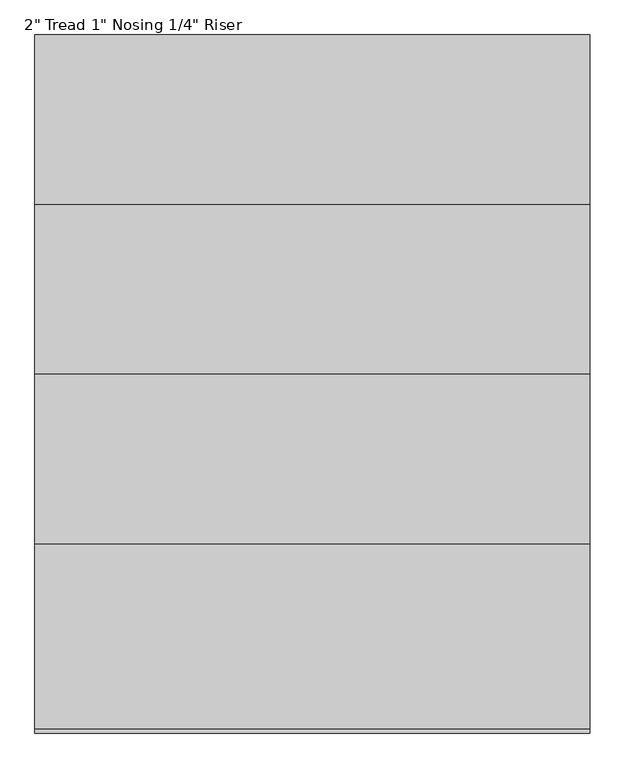
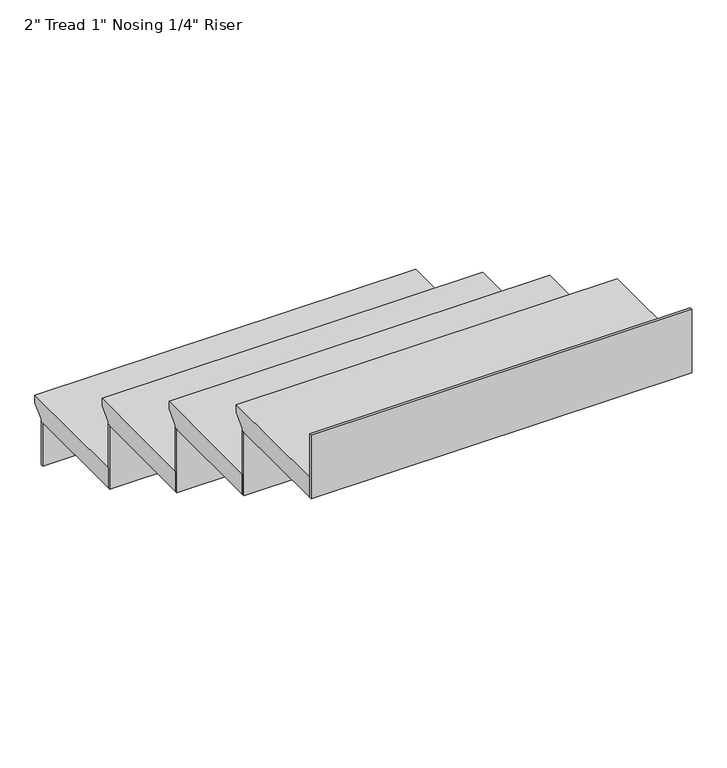
"""IFC4 building model written with IfcOpenShell, lengths in millimetres: stair flight geometry."""

from ifc_helpers import new_model, si_unit, origin, place, context, project, spatial, faceted_brep, source, transform, mapped, element, save


def stair_flight_6dcdbca7(model_context):
    return source(origin(), model_context, "Body", "Brep", [
        faceted_brep([(2695.3430349, 4115.4555142, 1415.3029412), (2695.3430349, 4115.4555142, 1434.3529412), (3609.7430349, 4115.4555142, 1434.3529412), (3609.7430349, 4115.4555142, 1415.3029412), (2695.3430349, 4090.0555142, 1389.9029412), (3609.7430349, 4090.0555142, 1389.9029412), (2695.3430349, 3810.6555142, 1434.3529412), (3609.7430349, 3810.6555142, 1434.3529412), (3609.7430349, 4090.0555142, 1383.5529412), (3609.7430349, 3810.6555142, 1383.5529412), (2695.3430349, 3810.6555142, 1383.5529412), (2695.3430349, 4090.0555142, 1383.5529412)], [[[0, 1, 2, 3]], [[4, 0, 3, 5]], [[2, 1, 6, 7]], [[8, 9, 10, 11]], [[2, 7, 9, 8, 5, 3]], [[8, 11, 4, 5]], [[6, 1, 0, 4, 11, 10]], [[7, 6, 10, 9]]]),
        faceted_brep([(2695.3430349, 4090.0555142, 1383.5529412), (2695.3430349, 4090.0555142, 1272.9882353), (2695.3430349, 4083.7055142, 1272.9882353), (2695.3430349, 4083.7055142, 1383.5529412), (3609.7430349, 4090.0555142, 1383.5529412), (3609.7430349, 4083.7055142, 1383.5529412), (3609.7430349, 4083.7055142, 1272.9882353), (3609.7430349, 4090.0555142, 1272.9882353)], [[[0, 1, 2, 3]], [[4, 5, 6, 7]], [[1, 0, 4, 7]], [[2, 1, 7, 6]], [[3, 2, 6, 5]], [[0, 3, 5, 4]]]),
        faceted_brep([(2695.3430349, 3810.6555142, 1544.9176471), (2695.3430349, 3810.6555142, 1383.5529412), (2695.3430349, 3804.3055142, 1383.5529412), (2695.3430349, 3804.3055142, 1544.9176471), (3609.7430349, 3810.6555142, 1544.9176471), (3609.7430349, 3804.3055142, 1544.9176471), (3609.7430349, 3804.3055142, 1383.5529412), (3609.7430349, 3810.6555142, 1383.5529412)], [[[0, 1, 2, 3]], [[4, 5, 6, 7]], [[1, 0, 4, 7]], [[2, 1, 7, 6]], [[3, 2, 6, 5]], [[0, 3, 5, 4]]]),
        faceted_brep([(3609.7430349, 3836.0555142, 1595.7176471), (2695.3430349, 3836.0555142, 1595.7176471), (2695.3430349, 3531.2555142, 1595.7176471), (3609.7430349, 3531.2555142, 1595.7176471), (3609.7430349, 3810.6555142, 1544.9176471), (3609.7430349, 3531.2555142, 1544.9176471), (2695.3430349, 3531.2555142, 1544.9176471), (2695.3430349, 3810.6555142, 1544.9176471), (3609.7430349, 3810.6555142, 1551.2676471), (3609.7430349, 3836.0555142, 1576.6676471), (2695.3430349, 3810.6555142, 1551.2676471), (2695.3430349, 3836.0555142, 1576.6676471)], [[[0, 1, 2, 3]], [[4, 5, 6, 7]], [[0, 3, 5, 4, 8, 9]], [[4, 7, 10, 8]], [[2, 1, 11, 10, 7, 6]], [[3, 2, 6, 5]], [[11, 1, 0, 9]], [[10, 11, 9, 8]]]),
        faceted_brep([(2695.3430349, 3531.2555142, 1706.2823529), (2695.3430349, 3531.2555142, 1544.9176471), (2695.3430349, 3524.9055142, 1544.9176471), (2695.3430349, 3524.9055142, 1706.2823529), (3609.7430349, 3531.2555142, 1706.2823529), (3609.7430349, 3524.9055142, 1706.2823529), (3609.7430349, 3524.9055142, 1544.9176471), (3609.7430349, 3531.2555142, 1544.9176471)], [[[0, 1, 2, 3]], [[4, 5, 6, 7]], [[1, 0, 4, 7]], [[2, 1, 7, 6]], [[3, 2, 6, 5]], [[0, 3, 5, 4]]]),
        faceted_brep([(3609.7430349, 3556.6555142, 1757.0823529), (2695.3430349, 3556.6555142, 1757.0823529), (2695.3430349, 3251.8555142, 1757.0823529), (3609.7430349, 3251.8555142, 1757.0823529), (3609.7430349, 3531.2555142, 1706.2823529), (3609.7430349, 3251.8555142, 1706.2823529), (2695.3430349, 3251.8555142, 1706.2823529), (2695.3430349, 3531.2555142, 1706.2823529), (3609.7430349, 3531.2555142, 1712.6323529), (3609.7430349, 3556.6555142, 1738.0323529), (2695.3430349, 3531.2555142, 1712.6323529), (2695.3430349, 3556.6555142, 1738.0323529)], [[[0, 1, 2, 3]], [[4, 5, 6, 7]], [[0, 3, 5, 4, 8, 9]], [[4, 7, 10, 8]], [[2, 1, 11, 10, 7, 6]], [[3, 2, 6, 5]], [[11, 1, 0, 9]], [[10, 11, 9, 8]]]),
        faceted_brep([(2695.3430349, 2972.4555142, 2029.0117647), (2695.3430349, 2972.4555142, 1867.6470588), (2695.3430349, 2966.1055142, 1867.6470588), (2695.3430349, 2966.1055142, 2029.0117647), (3609.7430349, 2972.4555142, 2029.0117647), (3609.7430349, 2966.1055142, 2029.0117647), (3609.7430349, 2966.1055142, 1867.6470588), (3609.7430349, 2972.4555142, 1867.6470588)], [[[0, 1, 2, 3]], [[4, 5, 6, 7]], [[1, 0, 4, 7]], [[2, 1, 7, 6]], [[3, 2, 6, 5]], [[0, 3, 5, 4]]]),
        faceted_brep([(2695.3430349, 3251.8555142, 1867.6470588), (2695.3430349, 3251.8555142, 1706.2823529), (2695.3430349, 3245.5055142, 1706.2823529), (2695.3430349, 3245.5055142, 1867.6470588), (3609.7430349, 3251.8555142, 1867.6470588), (3609.7430349, 3245.5055142, 1867.6470588), (3609.7430349, 3245.5055142, 1706.2823529), (3609.7430349, 3251.8555142, 1706.2823529)], [[[0, 1, 2, 3]], [[4, 5, 6, 7]], [[1, 0, 4, 7]], [[2, 1, 7, 6]], [[3, 2, 6, 5]], [[0, 3, 5, 4]]]),
        faceted_brep([(3609.7430349, 2972.4555142, 1918.4470588), (3609.7430349, 2997.8555142, 1918.4470588), (3609.7430349, 3277.2555142, 1918.4470588), (2695.3430349, 3277.2555142, 1918.4470588), (2695.3430349, 2972.4555142, 1918.4470588), (3609.7430349, 2997.8555142, 1867.6470588), (3609.7430349, 2972.4555142, 1867.6470588), (2695.3430349, 2972.4555142, 1867.6470588), (2695.3430349, 3251.8555142, 1867.6470588), (3609.7430349, 3251.8555142, 1867.6470588), (3609.7430349, 3251.8555142, 1873.9970588), (3609.7430349, 3277.2555142, 1899.3970588), (2695.3430349, 3251.8555142, 1873.9970588), (2695.3430349, 3277.2555142, 1899.3970588)], [[[0, 1, 2, 3, 4]], [[5, 6, 7, 8, 9]], [[1, 0, 6, 5]], [[2, 1, 5, 9, 10, 11]], [[9, 8, 12, 10]], [[4, 3, 13, 12, 8, 7]], [[0, 4, 7, 6]], [[13, 3, 2, 11]], [[12, 13, 11, 10]]]),
    ])


if __name__ == "__main__":
    model = new_model("IFC4")
    model_context = context("Model", 3, world=origin())
    ifc_project = project(units=[si_unit("LENGTHUNIT", "METRE", prefix="MILLI")], contexts=[model_context])
    site = spatial("IfcSite", under=ifc_project)
    building = spatial("IfcBuilding", under=site)
    placement = place(None, origin())
    stair_flight_shape = stair_flight_6dcdbca7(model_context)
    element("IfcStairFlight", 1, ObjectType="2\" Tread 1\" Nosing 1/4\" Riser", at=placement, inside=building, context=model_context, shape_type="MappedRepresentation", body=[
        mapped(stair_flight_shape, transform((0.0, 0.0, 0.0), x_axis=(1.0, 0.0, 0.0), y_axis=(0.0, 1.0, 0.0), z_axis=(0.0, 0.0, 1.0))),
    ])
    save(model, "model.ifc")
